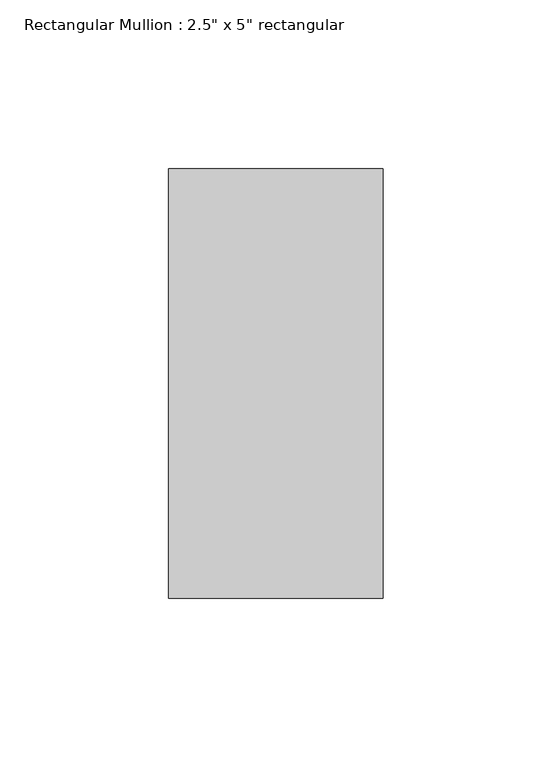
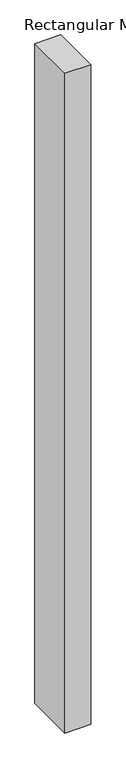
"""IFC4 building model written with IfcOpenShell, lengths in millimetres: member geometry."""

from ifc_helpers import new_model, si_unit, frame, origin, place, context, project, spatial, polyline, outline, extrude, source, transform, mapped, element, save


def member_7bc42366(model_context):
    return source(origin(), model_context, "Body", "SweptSolid", [
        extrude(outline(polyline([(0.0, 63.5), (0.0, -63.5), (-63.5, -63.5), (-63.5, 63.5), (0.0, 63.5)])), frame((0.0, 0.0, -1701.8), z_axis=(0.0, 0.0, 1.0), x_axis=(1.0, 0.0, 0.0)), (0.0, 0.0, 1.0), 1701.8),
    ])


if __name__ == "__main__":
    model = new_model("IFC4")
    model_context = context("Model", 3, world=origin())
    ifc_project = project(units=[si_unit("LENGTHUNIT", "METRE", prefix="MILLI")], contexts=[model_context])
    site = spatial("IfcSite", under=ifc_project)
    building = spatial("IfcBuilding", under=site)
    placement = place(None, origin())
    member_shape = member_7bc42366(model_context)
    element("IfcMember", 1, ObjectType="Rectangular Mullion : 2.5\" x 5\" rectangular", at=placement, inside=building, context=model_context, shape_type="MappedRepresentation", body=[
        mapped(member_shape, transform((0.0, 0.0, 0.0), x_axis=(1.0, 0.0, 0.0), y_axis=(0.0, 1.0, 0.0), z_axis=(0.0, 0.0, 1.0))),
    ])
    save(model, "model.ifc")

# Revit data of these elements
# Type "Rectangular Mullion : 2.5\" x 5\" rectangular"
#   built-in parameter 1007304 = 0.416667 (stored number, unit not read)
#   built-in parameter 1007301 = 0.104167 (stored number, unit not read)
#   built-in parameter 1007300 = 0.104167 (stored number, unit not read)
# Element 1 (IfcMember, "Rectangular Mullion : 2.5\" x 5\" rectangular")
#   Materials on its faces: "Iron, Ductile"
# Materials
#   "Iron, Ductile": class "Metal", colour RGB 0 0 0, transparency 0, Description = "Ductile cast iron", Cost = 0
